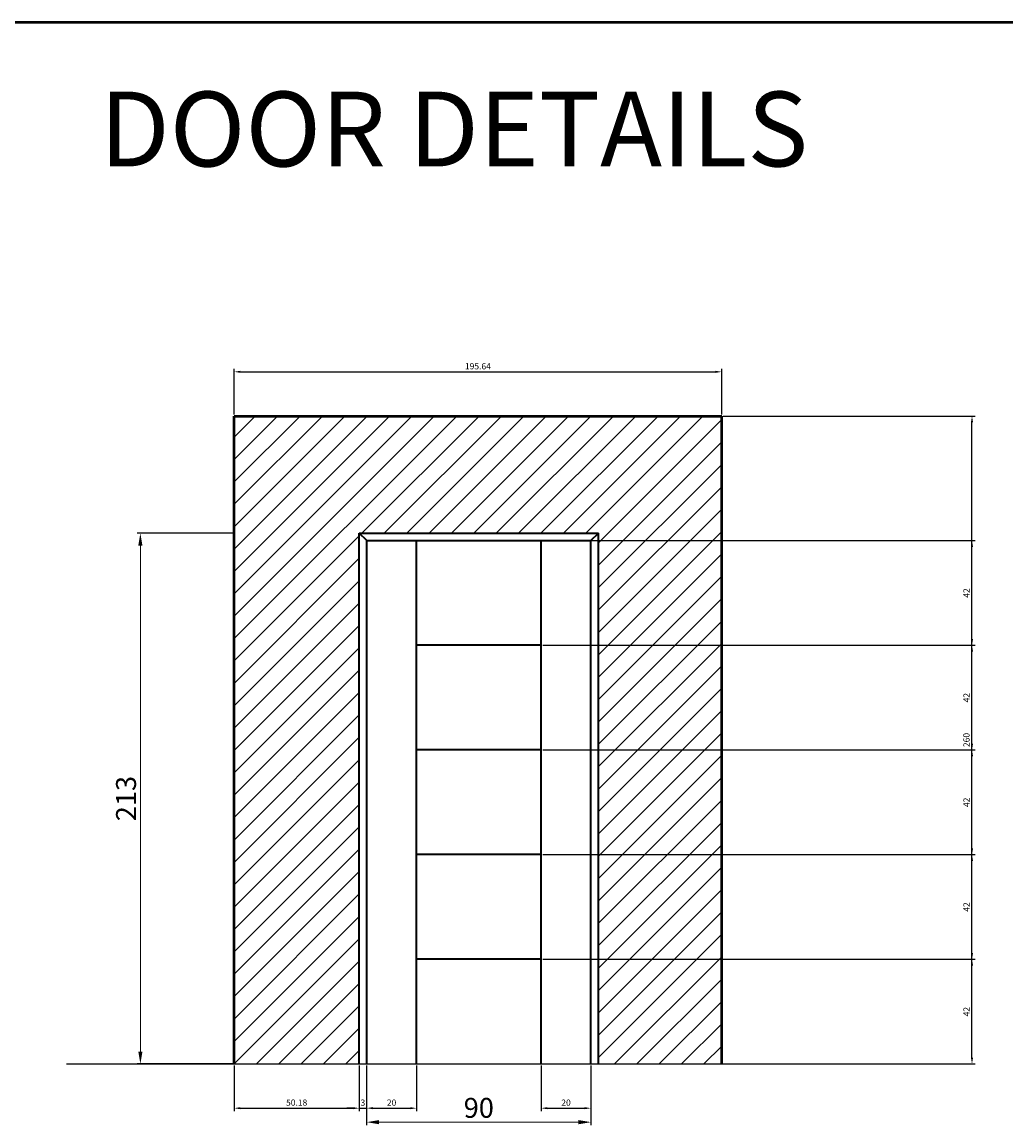
# Model space of a CAD drawing. Units: centimetres. Extents: x 1523 to 2760, y 1250 to 2134.
# Tile 3 of 4: x 1918 to 2313, y 1691 to 2134. Entities that reach past the tile are written whole.
import ezdxf

# ---------------------------------------------------------------- set-up
doc = ezdxf.new("R2010")
doc.units = ezdxf.units.CM
for name, color, linetype, lineweight in [('A-ANNO-DIMS', 2, 'Continuous', 18), ('A-ANNO-NPLT', 8, 'Continuous', 13), ('A-ANNO-TEXT', 7, 'Continuous', 18), ('A-ANNO-TTLB', 7, 'Continuous', 50), ('A-DOOR', 4, 'Continuous', 35), ('A-FLOR', 7, 'Continuous', 25), ('A-WALL', 7, 'Continuous', 50), ('A-WALL-PATT', 251, 'Continuous', 13)]:
    doc.layers.add(name, color=color, linetype=linetype, lineweight=lineweight)
doc.styles.get("Standard").update_dxf_attribs({"font": 'arial.ttf'})
doc.dimstyles.new('ISO-25', dxfattribs={"dimtxt": 2.5, "dimasz": 2.5, "dimexe": 1.25, "dimexo": 0.625, "dimtad": 1, "dimtxsty": 'Standard', "dimcen": 2.5, "dimadec": 0, "dimazin": 0, "dimtfac": 1, "dimtmove": 0, "dimatfit": 3, "dimfxl": 1, "dimarcsym": 0})

# ---------------------------------------------------------------- blocks, each defined once
blk = doc.blocks.new('*D4')
at = {"layer": 'A-ANNO-DIMS', "color": 0, "lineweight": -2, "transparency": 16777216}
for p, q in [((2002.51, 1928.7), (1964.27, 1928.7)), ((2002.51, 1715.7), (1964.27, 1715.7))]:
    blk.add_line(p, q, dxfattribs=at)
at = {"layer": 'A-ANNO-DIMS', "color": 0, "lineweight": 0, "transparency": 16777216}
blk.add_line((1965.52, 1720.7), (1965.52, 1923.7), dxfattribs=at)
at = {"layer": 'A-ANNO-DIMS', "color": 0, "transparency": 16777216}
for points in [[(1964.68, 1923.7), (1966.35, 1923.7), (1965.52, 1928.7)], [(1964.68, 1720.7), (1966.35, 1720.7), (1965.52, 1715.7)]]:
    blk.add_solid(points, dxfattribs=at)
at = {"layer": 'Defpoints', "color": 0, "transparency": 16777216}
for p in [(1965.52, 1928.7), (2003.14, 1928.7), (2003.14, 1715.7)]:
    blk.add_point(p, dxfattribs=at)
at = {"layer": 'A-ANNO-DIMS', "color": 0, "transparency": 16777216, "insert": (1960.8, 1822.2), "char_height": 8, "attachment_point": 5, "rotation": 90}
blk.add_mtext('213', dxfattribs=at)
blk = doc.blocks.new('*D5')
at = {"layer": 'A-ANNO-DIMS', "color": 0, "lineweight": -2, "transparency": 16777216}
for p, q in [((2056.32, 1715.08), (2056.32, 1691.09)), ((2146.32, 1715.08), (2146.32, 1691.09))]:
    blk.add_line(p, q, dxfattribs=at)
at = {"layer": 'A-ANNO-DIMS', "color": 0, "lineweight": 0, "transparency": 16777216}
blk.add_line((2061.32, 1692.34), (2141.32, 1692.34), dxfattribs=at)
at = {"layer": 'A-ANNO-DIMS', "color": 0, "transparency": 16777216}
for points in [[(2061.32, 1693.18), (2061.32, 1691.51), (2056.32, 1692.34)], [(2141.32, 1693.18), (2141.32, 1691.51), (2146.32, 1692.34)]]:
    blk.add_solid(points, dxfattribs=at)
at = {"layer": 'Defpoints', "color": 0, "transparency": 16777216}
for p in [(2056.32, 1715.7), (2146.32, 1715.7), (2146.32, 1692.34)]:
    blk.add_point(p, dxfattribs=at)
at = {"layer": 'A-ANNO-DIMS', "color": 0, "transparency": 16777216, "insert": (2101.32, 1697.05), "char_height": 8, "attachment_point": 5}
blk.add_mtext('90', dxfattribs=at)
blk = doc.blocks.new('*D17')
at = {"layer": 'A-ANNO-DIMS', "color": 0, "lineweight": -2, "transparency": 16777216}
for p, q in [((2003.14, 1976.33), (2003.14, 1994.7)), ((2005.64, 1993.45), (2196.28, 1993.45)), ((2198.78, 1976.33), (2198.78, 1994.7))]:
    blk.add_line(p, q, dxfattribs=at)
at = {"layer": 'A-ANNO-DIMS', "color": 0, "transparency": 16777216}
for points in [[(2005.64, 1993.87), (2005.64, 1993.04), (2003.14, 1993.45)], [(2196.28, 1993.87), (2196.28, 1993.04), (2198.78, 1993.45)]]:
    blk.add_solid(points, dxfattribs=at)
at = {"layer": 'Defpoints', "color": 0, "transparency": 16777216}
for p in [(2198.78, 1993.45), (2003.14, 1975.7), (2198.78, 1975.7)]:
    blk.add_point(p, dxfattribs=at)
at = {"layer": 'A-ANNO-DIMS', "color": 0, "transparency": 16777216, "insert": (2100.96, 1995.36), "char_height": 2.5, "attachment_point": 5}
blk.add_mtext('195.64', dxfattribs=at)
blk = doc.blocks.new('*D18')
at = {"layer": 'A-ANNO-DIMS', "color": 0, "lineweight": -2, "transparency": 16777216}
for p, q in [((2199.41, 1975.7), (2300.48, 1975.7)), ((2299.23, 1718.2), (2299.23, 1973.2)), ((2199.41, 1715.7), (2300.48, 1715.7))]:
    blk.add_line(p, q, dxfattribs=at)
at = {"layer": 'A-ANNO-DIMS', "color": 0, "transparency": 16777216}
for points in [[(2298.81, 1973.2), (2299.65, 1973.2), (2299.23, 1975.7)], [(2298.81, 1718.2), (2299.65, 1718.2), (2299.23, 1715.7)]]:
    blk.add_solid(points, dxfattribs=at)
at = {"layer": 'Defpoints', "color": 0, "transparency": 16777216}
for p in [(2198.78, 1975.7), (2299.23, 1975.7), (2198.78, 1715.7)]:
    blk.add_point(p, dxfattribs=at)
at = {"layer": 'A-ANNO-DIMS', "color": 0, "transparency": 16777216, "insert": (2297.33, 1845.7), "char_height": 2.5, "attachment_point": 5, "rotation": 90}
blk.add_mtext('260', dxfattribs=at)
blk = doc.blocks.new('*D19')
at = {"layer": 'A-ANNO-DIMS', "color": 0, "lineweight": -2, "transparency": 16777216}
for p, q in [((2053.32, 1715.08), (2053.32, 1696.7)), ((2056.32, 1715.08), (2056.32, 1696.7)), ((2050.82, 1697.95), (2048.32, 1697.95)), ((2053.32, 1697.95), (2056.32, 1697.95)), ((2058.82, 1697.95), (2061.32, 1697.95))]:
    blk.add_line(p, q, dxfattribs=at)
at = {"layer": 'A-ANNO-DIMS', "color": 0, "transparency": 16777216}
for points in [[(2050.82, 1698.37), (2050.82, 1697.54), (2053.32, 1697.95)], [(2058.82, 1698.37), (2058.82, 1697.54), (2056.32, 1697.95)]]:
    blk.add_solid(points, dxfattribs=at)
at = {"layer": 'Defpoints', "color": 0, "transparency": 16777216}
for p in [(2053.32, 1715.7), (2056.32, 1715.7), (2056.32, 1697.95)]:
    blk.add_point(p, dxfattribs=at)
at = {"layer": 'A-ANNO-DIMS', "color": 0, "transparency": 16777216, "insert": (2054.82, 1699.86), "char_height": 2.5, "attachment_point": 5}
blk.add_mtext('3', dxfattribs=at)
blk = doc.blocks.new('*D20')
at = {"layer": 'A-ANNO-DIMS', "color": 0, "lineweight": -2, "transparency": 16777216}
for p, q in [((2056.32, 1715.08), (2056.32, 1696.7)), ((2076.32, 1715.08), (2076.32, 1696.7)), ((2058.82, 1697.95), (2073.82, 1697.95))]:
    blk.add_line(p, q, dxfattribs=at)
at = {"layer": 'A-ANNO-DIMS', "color": 0, "transparency": 16777216}
for points in [[(2058.82, 1698.37), (2058.82, 1697.54), (2056.32, 1697.95)], [(2073.82, 1698.37), (2073.82, 1697.54), (2076.32, 1697.95)]]:
    blk.add_solid(points, dxfattribs=at)
at = {"layer": 'Defpoints', "color": 0, "transparency": 16777216}
for p in [(2056.32, 1715.7), (2076.32, 1715.7), (2076.32, 1697.95)]:
    blk.add_point(p, dxfattribs=at)
at = {"layer": 'A-ANNO-DIMS', "color": 0, "transparency": 16777216, "insert": (2066.32, 1699.86), "char_height": 2.5, "attachment_point": 5}
blk.add_mtext('20', dxfattribs=at)
blk = doc.blocks.new('*D21')
at = {"layer": 'A-ANNO-DIMS', "color": 0, "lineweight": -2, "transparency": 16777216}
for p, q in [((2126.32, 1715.08), (2126.32, 1696.7)), ((2146.32, 1715.08), (2146.32, 1696.7)), ((2128.82, 1697.95), (2143.82, 1697.95))]:
    blk.add_line(p, q, dxfattribs=at)
at = {"layer": 'A-ANNO-DIMS', "color": 0, "transparency": 16777216}
for points in [[(2128.82, 1698.37), (2128.82, 1697.54), (2126.32, 1697.95)], [(2143.82, 1698.37), (2143.82, 1697.54), (2146.32, 1697.95)]]:
    blk.add_solid(points, dxfattribs=at)
at = {"layer": 'Defpoints', "color": 0, "transparency": 16777216}
for p in [(2126.32, 1715.7), (2146.32, 1715.7), (2146.32, 1697.95)]:
    blk.add_point(p, dxfattribs=at)
at = {"layer": 'A-ANNO-DIMS', "color": 0, "transparency": 16777216, "insert": (2136.32, 1699.86), "char_height": 2.5, "attachment_point": 5}
blk.add_mtext('20', dxfattribs=at)
blk = doc.blocks.new('*D22')
at = {"layer": 'A-ANNO-DIMS', "color": 0, "lineweight": -2, "transparency": 16777216}
for p, q in [((2126.95, 1757.7), (2300.48, 1757.7)), ((2299.23, 1718.2), (2299.23, 1755.2)), ((2126.95, 1715.7), (2300.48, 1715.7))]:
    blk.add_line(p, q, dxfattribs=at)
at = {"layer": 'A-ANNO-DIMS', "color": 0, "transparency": 16777216}
for points in [[(2298.81, 1755.2), (2299.65, 1755.2), (2299.23, 1757.7)], [(2298.81, 1718.2), (2299.65, 1718.2), (2299.23, 1715.7)]]:
    blk.add_solid(points, dxfattribs=at)
at = {"layer": 'Defpoints', "color": 0, "transparency": 16777216}
for p in [(2126.32, 1757.7), (2299.23, 1757.7), (2126.32, 1715.7)]:
    blk.add_point(p, dxfattribs=at)
at = {"layer": 'A-ANNO-DIMS', "color": 0, "transparency": 16777216, "insert": (2297.35, 1736.7), "char_height": 2.5, "attachment_point": 5, "rotation": 90}
blk.add_mtext('42', dxfattribs=at)
blk = doc.blocks.new('*D23')
at = {"layer": 'A-ANNO-DIMS', "color": 0, "lineweight": -2, "transparency": 16777216}
for p, q in [((2126.95, 1799.7), (2300.48, 1799.7)), ((2299.23, 1760.2), (2299.23, 1797.2)), ((2126.95, 1757.7), (2300.48, 1757.7))]:
    blk.add_line(p, q, dxfattribs=at)
at = {"layer": 'A-ANNO-DIMS', "color": 0, "transparency": 16777216}
for points in [[(2298.81, 1797.2), (2299.65, 1797.2), (2299.23, 1799.7)], [(2298.81, 1760.2), (2299.65, 1760.2), (2299.23, 1757.7)]]:
    blk.add_solid(points, dxfattribs=at)
at = {"layer": 'Defpoints', "color": 0, "transparency": 16777216}
for p in [(2126.32, 1799.7), (2299.23, 1799.7), (2126.32, 1757.7)]:
    blk.add_point(p, dxfattribs=at)
at = {"layer": 'A-ANNO-DIMS', "color": 0, "transparency": 16777216, "insert": (2297.35, 1778.7), "char_height": 2.5, "attachment_point": 5, "rotation": 90}
blk.add_mtext('42', dxfattribs=at)
blk = doc.blocks.new('*D24')
at = {"layer": 'A-ANNO-DIMS', "color": 0, "lineweight": -2, "transparency": 16777216}
for p, q in [((2126.95, 1841.7), (2300.48, 1841.7)), ((2299.23, 1802.2), (2299.23, 1839.2)), ((2126.95, 1799.7), (2300.48, 1799.7))]:
    blk.add_line(p, q, dxfattribs=at)
at = {"layer": 'A-ANNO-DIMS', "color": 0, "transparency": 16777216}
for points in [[(2298.81, 1839.2), (2299.65, 1839.2), (2299.23, 1841.7)], [(2298.81, 1802.2), (2299.65, 1802.2), (2299.23, 1799.7)]]:
    blk.add_solid(points, dxfattribs=at)
at = {"layer": 'Defpoints', "color": 0, "transparency": 16777216}
for p in [(2126.32, 1841.7), (2299.23, 1841.7), (2126.32, 1799.7)]:
    blk.add_point(p, dxfattribs=at)
at = {"layer": 'A-ANNO-DIMS', "color": 0, "transparency": 16777216, "insert": (2297.35, 1820.7), "char_height": 2.5, "attachment_point": 5, "rotation": 90}
blk.add_mtext('42', dxfattribs=at)
blk = doc.blocks.new('*D25')
at = {"layer": 'A-ANNO-DIMS', "color": 0, "lineweight": -2, "transparency": 16777216}
for p, q in [((2126.95, 1883.7), (2300.48, 1883.7)), ((2299.23, 1844.2), (2299.23, 1881.2)), ((2126.95, 1841.7), (2300.48, 1841.7))]:
    blk.add_line(p, q, dxfattribs=at)
at = {"layer": 'A-ANNO-DIMS', "color": 0, "transparency": 16777216}
for points in [[(2298.81, 1881.2), (2299.65, 1881.2), (2299.23, 1883.7)], [(2298.81, 1844.2), (2299.65, 1844.2), (2299.23, 1841.7)]]:
    blk.add_solid(points, dxfattribs=at)
at = {"layer": 'Defpoints', "color": 0, "transparency": 16777216}
for p in [(2126.32, 1883.7), (2299.23, 1883.7), (2126.32, 1841.7)]:
    blk.add_point(p, dxfattribs=at)
at = {"layer": 'A-ANNO-DIMS', "color": 0, "transparency": 16777216, "insert": (2297.35, 1862.7), "char_height": 2.5, "attachment_point": 5, "rotation": 90}
blk.add_mtext('42', dxfattribs=at)
blk = doc.blocks.new('*D26')
at = {"layer": 'A-ANNO-DIMS', "color": 0, "lineweight": -2, "transparency": 16777216}
for p, q in [((2126.95, 1925.7), (2300.48, 1925.7)), ((2299.23, 1886.2), (2299.23, 1923.2)), ((2126.95, 1883.7), (2300.48, 1883.7))]:
    blk.add_line(p, q, dxfattribs=at)
at = {"layer": 'A-ANNO-DIMS', "color": 0, "transparency": 16777216}
for points in [[(2298.81, 1923.2), (2299.65, 1923.2), (2299.23, 1925.7)], [(2298.81, 1886.2), (2299.65, 1886.2), (2299.23, 1883.7)]]:
    blk.add_solid(points, dxfattribs=at)
at = {"layer": 'Defpoints', "color": 0, "transparency": 16777216}
for p in [(2126.32, 1925.7), (2299.23, 1925.7), (2126.32, 1883.7)]:
    blk.add_point(p, dxfattribs=at)
at = {"layer": 'A-ANNO-DIMS', "color": 0, "transparency": 16777216, "insert": (2297.35, 1904.7), "char_height": 2.5, "attachment_point": 5, "rotation": 90}
blk.add_mtext('42', dxfattribs=at)
blk = doc.blocks.new('*D27')
at = {"layer": 'A-ANNO-DIMS', "color": 0, "lineweight": -2, "transparency": 16777216}
for p, q in [((2003.14, 1715.08), (2003.14, 1696.7)), ((2053.32, 1715.08), (2053.32, 1696.7)), ((2005.64, 1697.95), (2050.82, 1697.95))]:
    blk.add_line(p, q, dxfattribs=at)
at = {"layer": 'A-ANNO-DIMS', "color": 0, "transparency": 16777216}
for points in [[(2005.64, 1698.37), (2005.64, 1697.54), (2003.14, 1697.95)], [(2050.82, 1698.37), (2050.82, 1697.54), (2053.32, 1697.95)]]:
    blk.add_solid(points, dxfattribs=at)
at = {"layer": 'Defpoints', "color": 0, "transparency": 16777216}
for p in [(2003.14, 1715.7), (2053.32, 1715.7), (2053.32, 1697.95)]:
    blk.add_point(p, dxfattribs=at)
at = {"layer": 'A-ANNO-DIMS', "color": 0, "transparency": 16777216, "insert": (2028.23, 1699.86), "char_height": 2.5, "attachment_point": 5}
blk.add_mtext('50.18', dxfattribs=at)

msp = doc.modelspace()

# ---------------------------------------------------------------- hatches: boundary and pattern name
at = {"layer": 'A-WALL-PATT'}
h = msp.add_hatch(dxfattribs=at)
h.set_pattern_fill('ANSI31', color=256, scale=2)
h.paths.add_polyline_path([(2198.7804, 1975.7048), (2003.1396, 1975.7048), (2003.1396, 1715.7048), (2053.3227, 1715.7048), (2053.3227, 1928.7048), (2149.3227, 1928.7048), (2149.3227, 1715.7048), (2198.7804, 1715.7048)])

# ---------------------------------------------------------------- linework, layer by layer
at = {"layer": 'A-ANNO-NPLT'}
for p in [(2126.3227, 1883.7048), (2126.3227, 1841.7048), (2126.3227, 1799.7048), (2126.3227, 1757.7048)]:
    msp.add_point(p, dxfattribs=at)
at = {"layer": 'A-ANNO-TTLB'}
msp.add_lwpolyline([(1523.2447, 2133.8046), (2759.5532, 2133.8046), (2759.5532, 1250.2097), (1523.2447, 1250.2097)], close=True, dxfattribs=at)
at = {"layer": 'A-DOOR'}
for p, q in [((2053.3227, 1715.7048), (2053.3227, 1928.7048)), ((2053.3227, 1928.7048), (2149.3227, 1928.7048)), ((2056.3227, 1925.7048), (2053.3227, 1928.7048)), ((2146.3227, 1925.7048), (2149.3227, 1928.7048)), ((2149.3227, 1715.7048), (2149.3227, 1928.7048)), ((2056.3227, 1715.7048), (2056.3227, 1925.7048)), ((2056.3227, 1925.7048), (2146.3227, 1925.7048)), ((2076.3227, 1715.7048), (2076.3227, 1925.7048)), ((2126.3227, 1715.7048), (2126.3227, 1925.7048)), ((2146.3227, 1715.7048), (2146.3227, 1925.7048)), ((2126.3227, 1883.7048), (2076.3227, 1883.7048)), ((2126.3227, 1841.7048), (2076.3227, 1841.7048)), ((2126.3227, 1799.7048), (2076.3227, 1799.7048)), ((2126.3227, 1757.7048), (2076.3227, 1757.7048))]:
    msp.add_line(p, q, dxfattribs=at)
at = {"layer": 'A-FLOR'}
msp.add_line((1935.8401, 1715.7048), (2281.481, 1715.7048), dxfattribs=at)
at = {"layer": 'A-WALL'}
for p, q in [((2003.1396, 1715.7048), (2003.1396, 1975.7048)), ((2003.1396, 1975.7048), (2198.7804, 1975.7048)), ((2198.7804, 1715.7048), (2198.7804, 1975.7048))]:
    msp.add_line(p, q, dxfattribs=at)

# ---------------------------------------------------------------- texts
at = {"layer": 'A-ANNO-TEXT', "insert": (1949.1512, 2105.8831), "char_height": 30, "attachment_point": 1}
msp.add_mtext_dynamic_manual_height_columns('{\\fArial Black|b0|i0|c0|p34;DOOR DETAILS}', width=532.741684, gutter_width=12.5, heights=[0], dxfattribs=at)

# ---------------------------------------------------------------- dimensions: what is measured, and where the dimension line sits
at = {"layer": 'A-ANNO-DIMS'}
for base, p1, p2, override, picture, middle in [((2198.7804, 1993.4548), (2003.1396, 1975.7048), (2198.7804, 1975.7048), {"dimdec": 2, "dimlfac": 1, "dimrnd": 0, "dimzin": 0, "dimdsep": 46, "dimlunit": 2}, '*D17', (2100.96, 1995.3562)), ((2053.3227, 1697.9548), (2003.1396, 1715.7048), (2053.3227, 1715.7048), {"dimdec": 2, "dimlfac": 1, "dimrnd": 0, "dimzin": 0, "dimdsep": 46, "dimlunit": 2}, '*D27', (2028.2311, 1699.8562)), ((2056.3227, 1697.9548), (2053.3227, 1715.7048), (2056.3227, 1715.7048), {"dimdec": 0, "dimlfac": 1, "dimrnd": 0, "dimzin": 0, "dimdsep": 46, "dimlunit": 2}, '*D19', (2054.8227, 1699.8571)), ((2146.3227, 1692.3421), (2056.3227, 1715.7048), (2146.3227, 1715.7048), {"dimtxt": 8, "dimasz": 5, "dimclrd": 0, "dimclre": 0, "dimclrt": 0, "dimlwd": 0}, '*D5', (2101.3227, 1697.0517)), ((2076.3227, 1697.9548), (2056.3227, 1715.7048), (2076.3227, 1715.7048), {"dimdec": 0, "dimlfac": 1, "dimrnd": 0, "dimzin": 0, "dimdsep": 46, "dimlunit": 2}, '*D20', (2066.3227, 1699.8562)), ((2146.3227, 1697.9548), (2126.3227, 1715.7048), (2146.3227, 1715.7048), {"dimdec": 0, "dimlfac": 1, "dimrnd": 0, "dimzin": 0, "dimdsep": 46, "dimlunit": 2}, '*D21', (2136.3227, 1699.8562))]:
    dim = msp.add_linear_dim(base=base, p1=p1, p2=p2, dimstyle='ISO-25', override=override, dxfattribs=at)
    dim.commit()
    dim.dimension.update_dxf_attribs({"geometry": picture, "text_midpoint": middle})
for base, p1, p2, override, picture, middle in [((2299.231, 1975.7048), (2198.7804, 1715.7048), (2198.7804, 1975.7048), {"dimdec": 0, "dimlfac": 1, "dimrnd": 0, "dimzin": 0, "dimdsep": 46, "dimlunit": 2}, '*D18', (2297.3296, 1845.7048)), ((1965.5161, 1928.7048), (2003.1396, 1715.7048), (2003.1396, 1928.7048), {"dimtxt": 8, "dimasz": 5, "dimclrd": 0, "dimclre": 0, "dimclrt": 0, "dimlwd": 0}, '*D4', (1960.8038, 1822.2048)), ((2299.231, 1925.7048), (2126.3227, 1883.7048), (2126.3227, 1925.7048), {"dimdec": 0, "dimlfac": 1, "dimrnd": 0, "dimzin": 0, "dimdsep": 46, "dimlunit": 2}, '*D26', (2297.3509, 1904.7048)), ((2299.231, 1883.7048), (2126.3227, 1841.7048), (2126.3227, 1883.7048), {"dimdec": 0, "dimlfac": 1, "dimrnd": 0, "dimzin": 0, "dimdsep": 46, "dimlunit": 2}, '*D25', (2297.3509, 1862.7048)), ((2299.231, 1841.7048), (2126.3227, 1799.7048), (2126.3227, 1841.7048), {"dimdec": 0, "dimlfac": 1, "dimrnd": 0, "dimzin": 0, "dimdsep": 46, "dimlunit": 2}, '*D24', (2297.3509, 1820.7048)), ((2299.231, 1799.7048), (2126.3227, 1757.7048), (2126.3227, 1799.7048), {"dimdec": 0, "dimlfac": 1, "dimrnd": 0, "dimzin": 0, "dimdsep": 46, "dimlunit": 2}, '*D23', (2297.3509, 1778.7048)), ((2299.231, 1757.7048), (2126.3227, 1715.7048), (2126.3227, 1757.7048), {"dimdec": 0, "dimlfac": 1, "dimrnd": 0, "dimzin": 0, "dimdsep": 46, "dimlunit": 2}, '*D22', (2297.3509, 1736.7048))]:
    dim = msp.add_linear_dim(base=base, p1=p1, p2=p2, angle=90, dimstyle='ISO-25', override=override, dxfattribs=at)
    dim.commit()
    dim.dimension.update_dxf_attribs({"geometry": picture, "text_midpoint": middle})

doc.saveas('drawing.dxf')
